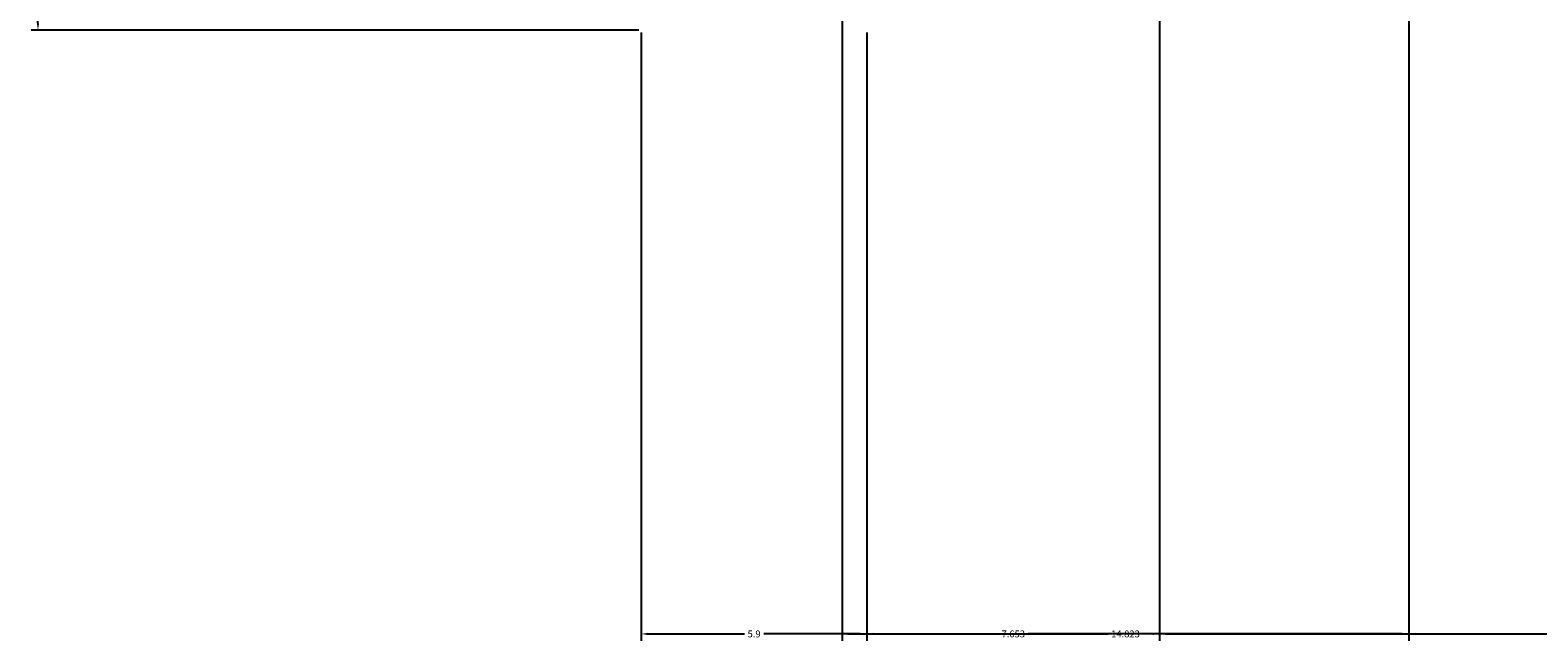
# Model space of a CAD drawing. Units: feet. Extents: x 2695 to 2912, y 795 to 1139.
# Tile 1 of 83: x 2695 to 2734, y 795 to 811. Entities that reach past the tile are written whole.
import ezdxf

# ---------------------------------------------------------------- set-up
doc = ezdxf.new("R2010")
doc.units = ezdxf.units.FT
doc.layers.add('A-ANNO-DIMS', color=2, linetype='Continuous', lineweight=18)
doc.styles.get("Standard").update_dxf_attribs({"font": 'arial.ttf'})
doc.dimstyles.get("Standard").update_dxf_attribs({"dimtxt": 0.18, "dimasz": 0.18, "dimexe": 0.18, "dimexo": 0.0625, "dimgap": 0.09, "dimtad": 0, "dimtih": 1, "dimtoh": 1, "dimdec": 1, "dimzin": 0, "dimdsep": 46, "dimlunit": 3, "dimtxsty": 'Standard', "dimcen": 0.09, "dimadec": 0, "dimazin": 0, "dimtfac": 1, "dimtdec": 1, "dimtofl": 0, "dimtmove": 0, "dimatfit": 3, "dimfxl": 1, "dimtolj": 1, "dimtzin": 0, "dimarcsym": 0})

# ---------------------------------------------------------------- blocks, each defined once
blk = doc.blocks.new('*D1')
at = {"layer": 'A-ANNO-DIMS', "color": 0, "lineweight": -2, "transparency": 16777216}
for p, q in [((2710.636, 810.868), (2710.636, 794.976)), ((2716.536, 810.868), (2716.536, 794.976)), ((2710.816, 795.156), (2713.332, 795.156)), ((2716.356, 795.156), (2713.84, 795.156))]:
    blk.add_line(p, q, dxfattribs=at)
at = {"layer": 'A-ANNO-DIMS', "color": 0, "transparency": 16777216}
for points in [[(2710.816, 795.186), (2710.816, 795.126), (2710.636, 795.156)], [(2716.356, 795.186), (2716.356, 795.126), (2716.536, 795.156)]]:
    blk.add_solid(points, dxfattribs=at)
at = {"layer": 'Defpoints', "color": 0, "transparency": 16777216}
for p in [(2710.636, 810.931), (2716.536, 810.931), (2716.536, 795.156)]:
    blk.add_point(p, dxfattribs=at)
at = {"layer": 'A-ANNO-DIMS', "color": 0, "transparency": 16777216, "insert": (2713.586, 795.156), "char_height": 0.18, "attachment_point": 5}
blk.add_mtext('\\A1;5.9', dxfattribs=at)
blk = doc.blocks.new('*D2')
at = {"layer": 'A-ANNO-DIMS', "color": 0, "lineweight": -2, "transparency": 16777216}
for p, q in [((2724.189, 874.795), (2724.189, 794.976)), ((2716.536, 810.868), (2716.536, 794.976)), ((2716.716, 795.156), (2719.97, 795.156)), ((2724.009, 795.156), (2720.756, 795.156))]:
    blk.add_line(p, q, dxfattribs=at)
at = {"layer": 'A-ANNO-DIMS', "color": 0, "transparency": 16777216}
for points in [[(2716.716, 795.186), (2716.716, 795.126), (2716.536, 795.156)], [(2724.009, 795.186), (2724.009, 795.126), (2724.189, 795.156)]]:
    blk.add_solid(points, dxfattribs=at)
at = {"layer": 'Defpoints', "color": 0, "transparency": 16777216}
for p in [(2724.189, 874.857), (2716.536, 810.931), (2724.189, 795.156)]:
    blk.add_point(p, dxfattribs=at)
at = {"layer": 'A-ANNO-DIMS', "color": 0, "transparency": 16777216, "insert": (2720.363, 795.156), "char_height": 0.18, "attachment_point": 5}
blk.add_mtext('\\A1;7.653', dxfattribs=at)
blk = doc.blocks.new('*D3')
at = {"layer": 'A-ANNO-DIMS', "color": 0, "lineweight": -2, "transparency": 16777216}
for p, q in [((2724.189, 874.795), (2724.189, 794.976)), ((2758.151, 874.795), (2758.151, 794.976)), ((2724.369, 795.156), (2740.777, 795.156)), ((2757.971, 795.156), (2741.564, 795.156))]:
    blk.add_line(p, q, dxfattribs=at)
at = {"layer": 'A-ANNO-DIMS', "color": 0, "transparency": 16777216}
for points in [[(2724.369, 795.186), (2724.369, 795.126), (2724.189, 795.156)], [(2757.971, 795.186), (2757.971, 795.126), (2758.151, 795.156)]]:
    blk.add_solid(points, dxfattribs=at)
at = {"layer": 'Defpoints', "color": 0, "transparency": 16777216}
for p in [(2724.189, 874.857), (2758.151, 874.857), (2758.151, 795.156)]:
    blk.add_point(p, dxfattribs=at)
at = {"layer": 'A-ANNO-DIMS', "color": 0, "transparency": 16777216, "insert": (2741.17, 795.156), "char_height": 0.18, "attachment_point": 5}
blk.add_mtext('\\A1;33.96', dxfattribs=at)
blk = doc.blocks.new('*D12')
at = {"layer": 'A-ANNO-DIMS', "color": 0, "lineweight": -2, "transparency": 16777216}
for p, q in [((2710.574, 1122.931), (2694.681, 1122.931)), ((2694.861, 1122.751), (2694.861, 967.113)), ((2694.861, 811.111), (2694.861, 966.749)), ((2710.574, 810.931), (2694.681, 810.931))]:
    blk.add_line(p, q, dxfattribs=at)
at = {"layer": 'A-ANNO-DIMS', "color": 0, "transparency": 16777216}
for points in [[(2694.831, 1122.751), (2694.891, 1122.751), (2694.861, 1122.931)], [(2694.831, 811.111), (2694.891, 811.111), (2694.861, 810.931)]]:
    blk.add_solid(points, dxfattribs=at)
at = {"layer": 'Defpoints', "color": 0, "transparency": 16777216}
for p in [(2694.861, 1122.931), (2710.636, 1122.931), (2710.636, 810.931)]:
    blk.add_point(p, dxfattribs=at)
at = {"layer": 'A-ANNO-DIMS', "color": 0, "transparency": 16777216, "insert": (2694.861, 966.931), "char_height": 0.18, "attachment_point": 5}
blk.add_mtext('\\A1;312', dxfattribs=at)
blk = doc.blocks.new('*D23')
at = {"layer": 'A-ANNO-DIMS', "color": 0, "lineweight": -2, "transparency": 16777216}
for p, q in [((2715.885, 936.868), (2715.885, 794.976)), ((2730.708, 936.868), (2730.708, 794.976)), ((2716.065, 795.156), (2722.842, 795.156)), ((2730.528, 795.156), (2723.752, 795.156))]:
    blk.add_line(p, q, dxfattribs=at)
at = {"layer": 'A-ANNO-DIMS', "color": 0, "transparency": 16777216}
for points in [[(2716.065, 795.186), (2716.065, 795.126), (2715.885, 795.156)], [(2730.528, 795.186), (2730.528, 795.126), (2730.708, 795.156)]]:
    blk.add_solid(points, dxfattribs=at)
at = {"layer": 'Defpoints', "color": 0, "transparency": 16777216}
for p in [(2715.885, 936.931), (2730.708, 936.931), (2730.708, 795.156)]:
    blk.add_point(p, dxfattribs=at)
at = {"layer": 'A-ANNO-DIMS', "color": 0, "transparency": 16777216, "insert": (2723.297, 795.156), "char_height": 0.18, "attachment_point": 5}
blk.add_mtext('\\A1;14.823', dxfattribs=at)
blk = doc.blocks.new('*D24')
at = {"layer": 'A-ANNO-DIMS', "color": 0, "lineweight": -2, "transparency": 16777216}
for p, q in [((2730.708, 936.868), (2730.708, 794.976)), ((2755.112, 936.868), (2755.112, 794.976)), ((2730.888, 795.156), (2742.446, 795.156)), ((2754.932, 795.156), (2743.375, 795.156))]:
    blk.add_line(p, q, dxfattribs=at)
at = {"layer": 'A-ANNO-DIMS', "color": 0, "transparency": 16777216}
for points in [[(2730.888, 795.186), (2730.888, 795.126), (2730.708, 795.156)], [(2754.932, 795.186), (2754.932, 795.126), (2755.112, 795.156)]]:
    blk.add_solid(points, dxfattribs=at)
at = {"layer": 'Defpoints', "color": 0, "transparency": 16777216}
for p in [(2730.708, 936.931), (2755.112, 936.931), (2755.112, 795.156)]:
    blk.add_point(p, dxfattribs=at)
at = {"layer": 'A-ANNO-DIMS', "color": 0, "transparency": 16777216, "insert": (2742.91, 795.156), "char_height": 0.18, "attachment_point": 5}
blk.add_mtext('\\A1;24.404', dxfattribs=at)

msp = doc.modelspace()

# ---------------------------------------------------------------- dimensions: what is measured, and where the dimension line sits
at = {"layer": 'A-ANNO-DIMS'}
dim = msp.add_linear_dim(base=(2694.8611, 1122.9306), p1=(2710.6361, 810.9306), p2=(2710.6361, 1122.9306), angle=90, dimstyle='Standard', override={"dimdec": 0, "dimlfac": 1, "dimrnd": 0, "dimzin": 0, "dimdsep": 46, "dimlunit": 2}, dxfattribs=at)
dim.commit()
dim.dimension.update_dxf_attribs({"geometry": '*D12', "text_midpoint": (2694.8611, 966.9306)})
for base, p1, p2, override, picture, middle in [((2730.7081, 795.1556), (2715.8852, 936.9306), (2730.7081, 936.9306), {"dimdec": 3, "dimlfac": 1, "dimrnd": 0, "dimzin": 0, "dimdsep": 46, "dimlunit": 2}, '*D23', (2723.2967, 795.1556)), ((2755.1125, 795.1556), (2730.7081, 936.9306), (2755.1125, 936.9306), {"dimdec": 3, "dimlfac": 1, "dimrnd": 0, "dimzin": 0, "dimdsep": 46, "dimlunit": 2}, '*D24', (2742.9103, 795.1556)), ((2724.18927, 795.15559), (2716.53582, 810.93059), (2724.18927, 874.85709), {"dimdec": 3, "dimlfac": 1, "dimrnd": 0, "dimzin": 0, "dimdsep": 46, "dimlunit": 2}, '*D2', (2720.36254, 795.15559)), ((2758.1515, 795.1556), (2724.1893, 874.8571), (2758.1515, 874.8571), {"dimdec": 2, "dimlfac": 1, "dimrnd": 0, "dimzin": 0, "dimdsep": 46, "dimlunit": 2}, '*D3', (2741.1704, 795.1556)), ((2716.5358, 795.1556), (2710.6361, 810.9306), (2716.5358, 810.9306), {"dimdec": 1, "dimlfac": 1, "dimrnd": 0, "dimzin": 0, "dimdsep": 46, "dimlunit": 2}, '*D1', (2713.5859, 795.1556))]:
    dim = msp.add_linear_dim(base=base, p1=p1, p2=p2, dimstyle='Standard', override=override, dxfattribs=at)
    dim.commit()
    dim.dimension.update_dxf_attribs({"geometry": picture, "text_midpoint": middle})

doc.saveas('drawing.dxf')
